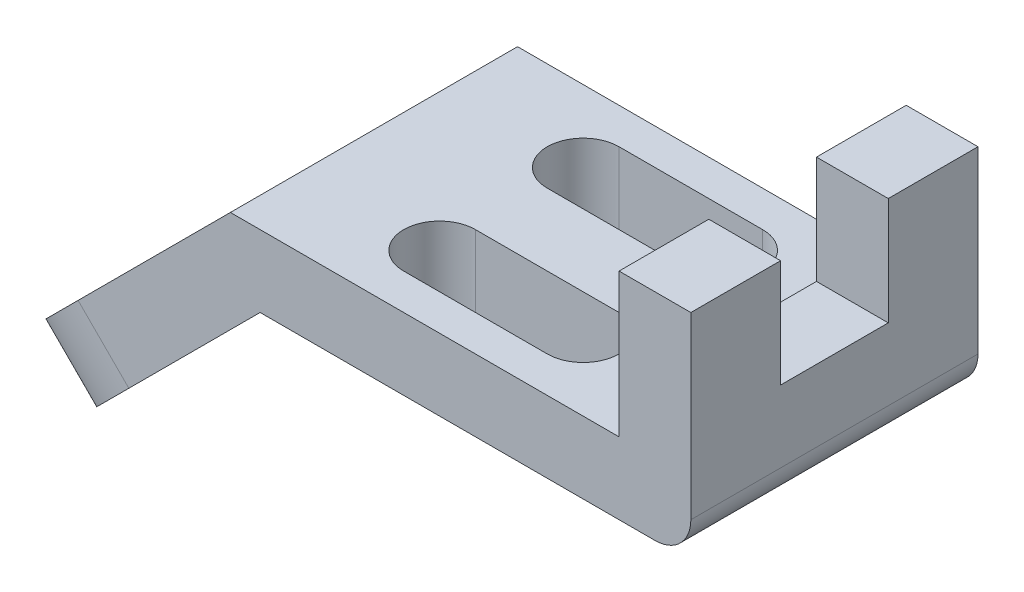
ISO-10303-21;
HEADER;
FILE_DESCRIPTION(('STEP AP214'),'2;1');
FILE_NAME('part.step','',(''),(''),'','','');
FILE_SCHEMA(('AUTOMOTIVE_DESIGN { 1 0 10303 214 1 1 1 1 }'));
ENDSEC;
DATA;
#1=APPLICATION_CONTEXT('core data for automotive mechanical design processes');
#2=APPLICATION_PROTOCOL_DEFINITION('international standard','automotive_design',2000,#1);
#3=PRODUCT_CONTEXT('',#1,'mechanical');
#4=PRODUCT('Part','Part','',(#3));
#5=PRODUCT_RELATED_PRODUCT_CATEGORY('part','',(#4));
#6=PRODUCT_DEFINITION_FORMATION('','',#4);
#7=PRODUCT_DEFINITION_CONTEXT('part definition',#1,'design');
#8=PRODUCT_DEFINITION('design','',#6,#7);
#9=PRODUCT_DEFINITION_SHAPE('','',#8);
#10=(LENGTH_UNIT() NAMED_UNIT(*) SI_UNIT(.MILLI.,.METRE.));
#11=(NAMED_UNIT(*) PLANE_ANGLE_UNIT() SI_UNIT($,.RADIAN.));
#12=(NAMED_UNIT(*) SI_UNIT($,.STERADIAN.) SOLID_ANGLE_UNIT());
#13=UNCERTAINTY_MEASURE_WITH_UNIT(LENGTH_MEASURE(1.E-05),#10,'distance_accuracy_value','');
#14=(GEOMETRIC_REPRESENTATION_CONTEXT(3) GLOBAL_UNCERTAINTY_ASSIGNED_CONTEXT((#13)) GLOBAL_UNIT_ASSIGNED_CONTEXT((#10,
#11,#12)) REPRESENTATION_CONTEXT('',''));
#15=CARTESIAN_POINT('',(0.,0.,0.));
#16=DIRECTION('',(0.,0.,1.));
#17=DIRECTION('',(1.,0.,0.));
#18=AXIS2_PLACEMENT_3D('',#15,#16,#17);
#19=CARTESIAN_POINT('',(-78.2842712474619,-18.2842712474619,0.));
#20=DIRECTION('',(-0.707106781186549,0.707106781186546,0.));
#21=DIRECTION('',(-0.707106781186546,-0.707106781186549,0.));
#22=AXIS2_PLACEMENT_3D('',#19,#20,#21);
#23=CYLINDRICAL_SURFACE('',#22,20.);
#24=DIRECTION('',(-0.707106781186549,0.707106781186546,0.));
#25=VECTOR('',#24,1.);
#26=CARTESIAN_POINT('',(-86.9558386639541,-26.9558386639541,15.7989821533687));
#27=LINE('',#26,#25);
#28=CARTESIAN_POINT('',(-86.9558386639541,-26.9558386639541,15.7989821533687));
#29=VERTEX_POINT('',#28);
#30=CARTESIAN_POINT('',(-94.0269064758195,-19.8847708520887,15.7989821533687));
#31=VERTEX_POINT('',#30);
#32=EDGE_CURVE('E50',#29,#31,#27,.T.);
#33=ORIENTED_EDGE('',*,*,#32,.F.);
#34=CARTESIAN_POINT('',(-78.2842712474619,-18.2842712474619,0.));
#35=DIRECTION('',(-0.707106781186549,0.707106781186546,0.));
#36=DIRECTION('',(-0.707106781186546,-0.707106781186549,0.));
#37=AXIS2_PLACEMENT_3D('',#34,#35,#36);
#38=CIRCLE('',#37,20.);
#39=CARTESIAN_POINT('',(-78.2842712474619,-18.2842712474619,20.));
#40=VERTEX_POINT('',#39);
#41=EDGE_CURVE('E325',#29,#40,#38,.T.);
#42=ORIENTED_EDGE('',*,*,#41,.T.);
#43=DIRECTION('',(0.707106781186547,-0.707106781186548,0.));
#44=VECTOR('',#43,1.);
#45=CARTESIAN_POINT('',(-85.3553390593273,-11.2132034355965,20.));
#46=LINE('',#45,#44);
#47=CARTESIAN_POINT('',(-85.3553390593273,-11.2132034355965,20.));
#48=VERTEX_POINT('',#47);
#49=EDGE_CURVE('E333',#48,#40,#46,.T.);
#50=ORIENTED_EDGE('',*,*,#49,.F.);
#51=CARTESIAN_POINT('',(-85.3553390593274,-11.2132034355965,0.));
#52=DIRECTION('',(-0.707106781186549,0.707106781186546,0.));
#53=DIRECTION('',(-0.707106781186546,-0.707106781186549,0.));
#54=AXIS2_PLACEMENT_3D('',#51,#52,#53);
#55=CIRCLE('',#54,20.);
#56=EDGE_CURVE('E320',#31,#48,#55,.T.);
#57=ORIENTED_EDGE('',*,*,#56,.F.);
#58=EDGE_LOOP('',(#33,#42,#50,#57));
#59=FACE_BOUND('',#58,.T.);
#60=ADVANCED_FACE('F39',(#59),#23,.T.);
#61=CARTESIAN_POINT('',(0.,30.,20.));
#62=DIRECTION('',(0.,-1.,0.));
#63=DIRECTION('',(0.,0.,-1.));
#64=AXIS2_PLACEMENT_3D('',#61,#62,#63);
#65=PLANE('',#64);
#66=DIRECTION('',(0.,0.,-1.));
#67=VECTOR('',#66,1.);
#68=CARTESIAN_POINT('',(-10.,30.,20.));
#69=LINE('',#68,#67);
#70=CARTESIAN_POINT('',(-10.,30.,-7.5));
#71=VERTEX_POINT('',#70);
#72=CARTESIAN_POINT('',(-10.,30.,-20.));
#73=VERTEX_POINT('',#72);
#74=EDGE_CURVE('E383',#71,#73,#69,.T.);
#75=ORIENTED_EDGE('',*,*,#74,.F.);
#76=DIRECTION('',(-1.,0.,0.));
#77=VECTOR('',#76,1.);
#78=CARTESIAN_POINT('',(0.001000000000001,30.,-7.5));
#79=LINE('',#78,#77);
#80=CARTESIAN_POINT('',(0.,30.,-7.5));
#81=VERTEX_POINT('',#80);
#82=EDGE_CURVE('E308',#81,#71,#79,.T.);
#83=ORIENTED_EDGE('',*,*,#82,.F.);
#84=DIRECTION('',(0.,0.,-1.));
#85=VECTOR('',#84,1.);
#86=CARTESIAN_POINT('',(0.,30.,20.));
#87=LINE('',#86,#85);
#88=CARTESIAN_POINT('',(0.,30.,-20.));
#89=VERTEX_POINT('',#88);
#90=EDGE_CURVE('E347',#81,#89,#87,.T.);
#91=ORIENTED_EDGE('',*,*,#90,.T.);
#92=DIRECTION('',(-1.,0.,0.));
#93=VECTOR('',#92,1.);
#94=CARTESIAN_POINT('',(0.,30.,-20.));
#95=LINE('',#94,#93);
#96=EDGE_CURVE('E321',#89,#73,#95,.T.);
#97=ORIENTED_EDGE('',*,*,#96,.T.);
#98=EDGE_LOOP('',(#75,#83,#91,#97));
#99=FACE_BOUND('',#98,.T.);
#100=ADVANCED_FACE('F460',(#99),#65,.F.);
#101=CARTESIAN_POINT('',(0.,30.,20.));
#102=VERTEX_POINT('',#101);
#103=CARTESIAN_POINT('',(0.,30.,7.5));
#104=VERTEX_POINT('',#103);
#105=EDGE_CURVE('E368',#102,#104,#87,.T.);
#106=ORIENTED_EDGE('',*,*,#105,.T.);
#107=DIRECTION('',(-1.,0.,0.));
#108=VECTOR('',#107,1.);
#109=CARTESIAN_POINT('',(0.001000000000001,30.,7.5));
#110=LINE('',#109,#108);
#111=CARTESIAN_POINT('',(-10.,30.,7.5));
#112=VERTEX_POINT('',#111);
#113=EDGE_CURVE('E310',#104,#112,#110,.T.);
#114=ORIENTED_EDGE('',*,*,#113,.T.);
#115=CARTESIAN_POINT('',(-10.,30.,20.));
#116=VERTEX_POINT('',#115);
#117=EDGE_CURVE('E384',#116,#112,#69,.T.);
#118=ORIENTED_EDGE('',*,*,#117,.F.);
#119=DIRECTION('',(-1.,0.,0.));
#120=VECTOR('',#119,1.);
#121=CARTESIAN_POINT('',(0.,30.,20.));
#122=LINE('',#121,#120);
#123=EDGE_CURVE('E322',#102,#116,#122,.T.);
#124=ORIENTED_EDGE('',*,*,#123,.F.);
#125=EDGE_LOOP('',(#106,#114,#118,#124));
#126=FACE_BOUND('',#125,.T.);
#127=ADVANCED_FACE('F41',(#126),#65,.F.);
#128=CARTESIAN_POINT('',(-10.,30.,20.));
#129=DIRECTION('',(1.,0.,0.));
#130=DIRECTION('',(0.,1.,0.));
#131=AXIS2_PLACEMENT_3D('',#128,#129,#130);
#132=PLANE('',#131);
#133=DIRECTION('',(0.,0.,1.));
#134=VECTOR('',#133,1.);
#135=CARTESIAN_POINT('',(-10.,15.,-7.5));
#136=LINE('',#135,#134);
#137=CARTESIAN_POINT('',(-10.,15.,-7.5));
#138=VERTEX_POINT('',#137);
#139=CARTESIAN_POINT('',(-10.,15.,7.5));
#140=VERTEX_POINT('',#139);
#141=EDGE_CURVE('E296',#138,#140,#136,.T.);
#142=ORIENTED_EDGE('',*,*,#141,.F.);
#143=DIRECTION('',(0.,-1.,0.));
#144=VECTOR('',#143,1.);
#145=CARTESIAN_POINT('',(-10.,30.,-7.5));
#146=LINE('',#145,#144);
#147=EDGE_CURVE('E299',#71,#138,#146,.T.);
#148=ORIENTED_EDGE('',*,*,#147,.F.);
#149=ORIENTED_EDGE('',*,*,#74,.T.);
#150=DIRECTION('',(0.,-1.,0.));
#151=VECTOR('',#150,1.);
#152=CARTESIAN_POINT('',(-10.,30.,-20.));
#153=LINE('',#152,#151);
#154=CARTESIAN_POINT('',(-10.,10.,-20.));
#155=VERTEX_POINT('',#154);
#156=EDGE_CURVE('E349',#73,#155,#153,.T.);
#157=ORIENTED_EDGE('',*,*,#156,.T.);
#158=DIRECTION('',(0.,0.,-1.));
#159=VECTOR('',#158,1.);
#160=CARTESIAN_POINT('',(-10.,10.,20.));
#161=LINE('',#160,#159);
#162=CARTESIAN_POINT('',(-10.,10.,20.));
#163=VERTEX_POINT('',#162);
#164=EDGE_CURVE('E381',#163,#155,#161,.T.);
#165=ORIENTED_EDGE('',*,*,#164,.F.);
#166=DIRECTION('',(0.,-1.,0.));
#167=VECTOR('',#166,1.);
#168=CARTESIAN_POINT('',(-10.,30.,20.));
#169=LINE('',#168,#167);
#170=EDGE_CURVE('E330',#116,#163,#169,.T.);
#171=ORIENTED_EDGE('',*,*,#170,.F.);
#172=ORIENTED_EDGE('',*,*,#117,.T.);
#173=DIRECTION('',(0.,1.,0.));
#174=VECTOR('',#173,1.);
#175=CARTESIAN_POINT('',(-10.,30.,7.5));
#176=LINE('',#175,#174);
#177=EDGE_CURVE('E303',#140,#112,#176,.T.);
#178=ORIENTED_EDGE('',*,*,#177,.F.);
#179=EDGE_LOOP('',(#142,#148,#149,#157,#165,#171,#172,#178));
#180=FACE_BOUND('',#179,.T.);
#181=ADVANCED_FACE('F429',(#180),#132,.F.);
#182=CARTESIAN_POINT('',(-10.,10.,20.));
#183=DIRECTION('',(0.,-1.,0.));
#184=DIRECTION('',(1.,0.,0.));
#185=AXIS2_PLACEMENT_3D('',#182,#183,#184);
#186=PLANE('',#185);
#187=DIRECTION('',(1.,0.,0.));
#188=VECTOR('',#187,1.);
#189=CARTESIAN_POINT('',(-45.,10.,-4.99999999999999));
#190=LINE('',#189,#188);
#191=CARTESIAN_POINT('',(-45.,9.99999999999999,-4.99999999999999));
#192=VERTEX_POINT('',#191);
#193=CARTESIAN_POINT('',(-25.,10.,-4.99999999999999));
#194=VERTEX_POINT('',#193);
#195=EDGE_CURVE('E245',#192,#194,#190,.T.);
#196=ORIENTED_EDGE('',*,*,#195,.F.);
#197=CARTESIAN_POINT('',(-45.,10.,-9.99999999999999));
#198=DIRECTION('',(0.,1.,0.));
#199=DIRECTION('',(-1.,0.,0.));
#200=AXIS2_PLACEMENT_3D('',#197,#198,#199);
#201=CIRCLE('',#200,5.);
#202=CARTESIAN_POINT('',(-45.,10.,-15.));
#203=VERTEX_POINT('',#202);
#204=EDGE_CURVE('E64',#203,#192,#201,.T.);
#205=ORIENTED_EDGE('',*,*,#204,.F.);
#206=DIRECTION('',(-1.,0.,0.));
#207=VECTOR('',#206,1.);
#208=CARTESIAN_POINT('',(-45.,10.,-15.));
#209=LINE('',#208,#207);
#210=CARTESIAN_POINT('',(-25.,10.,-15.));
#211=VERTEX_POINT('',#210);
#212=EDGE_CURVE('E246',#211,#203,#209,.T.);
#213=ORIENTED_EDGE('',*,*,#212,.F.);
#214=CARTESIAN_POINT('',(-25.,10.,-9.99999999999999));
#215=DIRECTION('',(0.,1.,0.));
#216=DIRECTION('',(-1.,0.,0.));
#217=AXIS2_PLACEMENT_3D('',#214,#215,#216);
#218=CIRCLE('',#217,5.);
#219=EDGE_CURVE('E250',#194,#211,#218,.T.);
#220=ORIENTED_EDGE('',*,*,#219,.F.);
#221=EDGE_LOOP('',(#196,#205,#213,#220));
#222=FACE_BOUND('',#221,.T.);
#223=DIRECTION('',(1.,0.,0.));
#224=VECTOR('',#223,1.);
#225=CARTESIAN_POINT('',(-45.,10.,15.));
#226=LINE('',#225,#224);
#227=CARTESIAN_POINT('',(-45.,9.99999999999999,15.));
#228=VERTEX_POINT('',#227);
#229=CARTESIAN_POINT('',(-25.,10.,15.));
#230=VERTEX_POINT('',#229);
#231=EDGE_CURVE('E273',#228,#230,#226,.T.);
#232=ORIENTED_EDGE('',*,*,#231,.F.);
#233=CARTESIAN_POINT('',(-45.,10.,9.99999999999999));
#234=DIRECTION('',(0.,1.,0.));
#235=DIRECTION('',(1.,0.,0.));
#236=AXIS2_PLACEMENT_3D('',#233,#234,#235);
#237=CIRCLE('',#236,5.);
#238=CARTESIAN_POINT('',(-45.,10.,4.99999999999999));
#239=VERTEX_POINT('',#238);
#240=EDGE_CURVE('E275',#239,#228,#237,.T.);
#241=ORIENTED_EDGE('',*,*,#240,.F.);
#242=DIRECTION('',(-1.,0.,0.));
#243=VECTOR('',#242,1.);
#244=CARTESIAN_POINT('',(-45.,10.,4.99999999999999));
#245=LINE('',#244,#243);
#246=CARTESIAN_POINT('',(-25.,10.,4.99999999999999));
#247=VERTEX_POINT('',#246);
#248=EDGE_CURVE('E278',#247,#239,#245,.T.);
#249=ORIENTED_EDGE('',*,*,#248,.F.);
#250=CARTESIAN_POINT('',(-25.,10.,9.99999999999999));
#251=DIRECTION('',(0.,1.,0.));
#252=DIRECTION('',(1.,0.,0.));
#253=AXIS2_PLACEMENT_3D('',#250,#251,#252);
#254=CIRCLE('',#253,5.);
#255=EDGE_CURVE('E280',#230,#247,#254,.T.);
#256=ORIENTED_EDGE('',*,*,#255,.F.);
#257=EDGE_LOOP('',(#232,#241,#249,#256));
#258=FACE_BOUND('',#257,.T.);
#259=DIRECTION('',(-1.,0.,0.));
#260=VECTOR('',#259,1.);
#261=CARTESIAN_POINT('',(-10.,10.,-20.));
#262=LINE('',#261,#260);
#263=CARTESIAN_POINT('',(-64.142135623731,9.99999999999999,-20.));
#264=VERTEX_POINT('',#263);
#265=EDGE_CURVE('E353',#155,#264,#262,.T.);
#266=ORIENTED_EDGE('',*,*,#265,.T.);
#267=DIRECTION('',(0.,0.,-1.));
#268=VECTOR('',#267,1.);
#269=CARTESIAN_POINT('',(-64.142135623731,9.99999999999999,20.));
#270=LINE('',#269,#268);
#271=CARTESIAN_POINT('',(-64.142135623731,9.99999999999999,20.));
#272=VERTEX_POINT('',#271);
#273=EDGE_CURVE('E378',#272,#264,#270,.T.);
#274=ORIENTED_EDGE('',*,*,#273,.F.);
#275=DIRECTION('',(-1.,0.,0.));
#276=VECTOR('',#275,1.);
#277=CARTESIAN_POINT('',(-10.,10.,20.));
#278=LINE('',#277,#276);
#279=EDGE_CURVE('E329',#163,#272,#278,.T.);
#280=ORIENTED_EDGE('',*,*,#279,.F.);
#281=ORIENTED_EDGE('',*,*,#164,.T.);
#282=EDGE_LOOP('',(#266,#274,#280,#281));
#283=FACE_BOUND('',#282,.T.);
#284=ADVANCED_FACE('F432',(#222,#258,#283),#186,.F.);
#285=CARTESIAN_POINT('',(-64.142135623731,9.99999999999999,20.));
#286=DIRECTION('',(0.707106781186549,-0.707106781186546,0.));
#287=DIRECTION('',(0.707106781186546,0.707106781186549,0.));
#288=AXIS2_PLACEMENT_3D('',#285,#286,#287);
#289=PLANE('',#288);
#290=CARTESIAN_POINT('',(-85.3553390593274,-11.2132034355965,0.));
#291=DIRECTION('',(-0.707106781186549,0.707106781186546,0.));
#292=DIRECTION('',(-0.707106781186546,-0.707106781186549,0.));
#293=AXIS2_PLACEMENT_3D('',#290,#291,#292);
#294=CIRCLE('',#293,12.5);
#295=CARTESIAN_POINT('',(-90.2290634162853,-16.0869277925544,10.4280209908108));
#296=VERTEX_POINT('',#295);
#297=CARTESIAN_POINT('',(-92.7290634162853,-18.5869277925544,6.89248708487803));
#298=VERTEX_POINT('',#297);
#299=EDGE_CURVE('E212',#296,#298,#294,.T.);
#300=ORIENTED_EDGE('',*,*,#299,.F.);
#301=DIRECTION('',(0.499999999999998,0.5,-0.707106781186549));
#302=VECTOR('',#301,1.);
#303=CARTESIAN_POINT('',(-90.2290634162853,-16.0869277925544,10.4280209908108));
#304=LINE('',#303,#302);
#305=EDGE_CURVE('E211',#31,#296,#304,.T.);
#306=ORIENTED_EDGE('',*,*,#305,.F.);
#307=ORIENTED_EDGE('',*,*,#56,.T.);
#308=DIRECTION('',(-0.707106781186546,-0.707106781186549,0.));
#309=VECTOR('',#308,1.);
#310=CARTESIAN_POINT('',(-64.142135623731,9.99999999999999,20.));
#311=LINE('',#310,#309);
#312=EDGE_CURVE('E335',#272,#48,#311,.T.);
#313=ORIENTED_EDGE('',*,*,#312,.F.);
#314=ORIENTED_EDGE('',*,*,#273,.T.);
#315=DIRECTION('',(-0.707106781186546,-0.707106781186549,0.));
#316=VECTOR('',#315,1.);
#317=CARTESIAN_POINT('',(-64.142135623731,9.99999999999999,-20.));
#318=LINE('',#317,#316);
#319=CARTESIAN_POINT('',(-85.3553390593273,-11.2132034355965,-20.));
#320=VERTEX_POINT('',#319);
#321=EDGE_CURVE('E352',#264,#320,#318,.T.);
#322=ORIENTED_EDGE('',*,*,#321,.T.);
#323=CARTESIAN_POINT('',(-96.5269064758195,-22.3847708520887,12.2634482474359));
#324=VERTEX_POINT('',#323);
#325=EDGE_CURVE('E221',#320,#324,#55,.T.);
#326=ORIENTED_EDGE('',*,*,#325,.T.);
#327=DIRECTION('',(-0.499999999999999,-0.5,0.707106781186549));
#328=VECTOR('',#327,1.);
#329=CARTESIAN_POINT('',(-92.7290634162853,-18.5869277925544,6.89248708487803));
#330=LINE('',#329,#328);
#331=EDGE_CURVE('E53',#298,#324,#330,.T.);
#332=ORIENTED_EDGE('',*,*,#331,.F.);
#333=EDGE_LOOP('',(#300,#306,#307,#313,#314,#322,#326,#332));
#334=FACE_BOUND('',#333,.T.);
#335=ADVANCED_FACE('F225',(#334),#289,.F.);
#336=CARTESIAN_POINT('',(-78.2842712474619,-18.2842712474619,20.));
#337=DIRECTION('',(-0.707106781186548,0.707106781186547,0.));
#338=DIRECTION('',(-0.707106781186547,-0.707106781186548,0.));
#339=AXIS2_PLACEMENT_3D('',#336,#337,#338);
#340=PLANE('',#339);
#341=ORIENTED_EDGE('',*,*,#41,.F.);
#342=DIRECTION('',(0.499999999999998,0.499999999999999,-0.707106781186549));
#343=VECTOR('',#342,1.);
#344=CARTESIAN_POINT('',(-84.1053390593273,-24.1053390593274,11.7677669529664));
#345=LINE('',#344,#343);
#346=CARTESIAN_POINT('',(-83.1579956044198,-23.1579956044199,10.4280209908108));
#347=VERTEX_POINT('',#346);
#348=EDGE_CURVE('E226',#29,#347,#345,.T.);
#349=ORIENTED_EDGE('',*,*,#348,.T.);
#350=CARTESIAN_POINT('',(-78.2842712474619,-18.2842712474619,0.));
#351=DIRECTION('',(-0.707106781186548,0.707106781186547,0.));
#352=DIRECTION('',(-0.707106781186547,-0.707106781186548,0.));
#353=AXIS2_PLACEMENT_3D('',#350,#351,#352);
#354=CIRCLE('',#353,12.5);
#355=CARTESIAN_POINT('',(-85.6579956044198,-25.6579956044199,6.89248708487803));
#356=VERTEX_POINT('',#355);
#357=EDGE_CURVE('E11',#347,#356,#354,.T.);
#358=ORIENTED_EDGE('',*,*,#357,.T.);
#359=DIRECTION('',(-0.499999999999999,-0.5,0.707106781186549));
#360=VECTOR('',#359,1.);
#361=CARTESIAN_POINT('',(-86.6053390593273,-26.6053390593274,8.23223304703367));
#362=LINE('',#361,#360);
#363=CARTESIAN_POINT('',(-89.4558386639541,-29.4558386639542,12.2634482474359));
#364=VERTEX_POINT('',#363);
#365=EDGE_CURVE('E208',#356,#364,#362,.T.);
#366=ORIENTED_EDGE('',*,*,#365,.T.);
#367=CARTESIAN_POINT('',(-78.2842712474619,-18.2842712474619,-20.));
#368=VERTEX_POINT('',#367);
#369=EDGE_CURVE('E318',#368,#364,#38,.T.);
#370=ORIENTED_EDGE('',*,*,#369,.F.);
#371=DIRECTION('',(0.707106781186547,0.707106781186548,0.));
#372=VECTOR('',#371,1.);
#373=CARTESIAN_POINT('',(-78.2842712474619,-18.2842712474619,-20.));
#374=LINE('',#373,#372);
#375=CARTESIAN_POINT('',(-60.,0.,-20.));
#376=VERTEX_POINT('',#375);
#377=EDGE_CURVE('E358',#368,#376,#374,.T.);
#378=ORIENTED_EDGE('',*,*,#377,.T.);
#379=DIRECTION('',(0.,0.,-1.));
#380=VECTOR('',#379,1.);
#381=CARTESIAN_POINT('',(-60.,0.,20.));
#382=LINE('',#381,#380);
#383=CARTESIAN_POINT('',(-60.,0.,20.));
#384=VERTEX_POINT('',#383);
#385=EDGE_CURVE('E374',#384,#376,#382,.T.);
#386=ORIENTED_EDGE('',*,*,#385,.F.);
#387=DIRECTION('',(0.707106781186547,0.707106781186548,0.));
#388=VECTOR('',#387,1.);
#389=CARTESIAN_POINT('',(-78.2842712474619,-18.2842712474619,20.));
#390=LINE('',#389,#388);
#391=EDGE_CURVE('E337',#40,#384,#390,.T.);
#392=ORIENTED_EDGE('',*,*,#391,.F.);
#393=EDGE_LOOP('',(#341,#349,#358,#366,#370,#378,#386,#392));
#394=FACE_BOUND('',#393,.T.);
#395=ADVANCED_FACE('F405',(#394),#340,.F.);
#396=CARTESIAN_POINT('',(-60.,0.,20.));
#397=DIRECTION('',(0.,1.,0.));
#398=DIRECTION('',(0.,0.,1.));
#399=AXIS2_PLACEMENT_3D('',#396,#397,#398);
#400=PLANE('',#399);
#401=DIRECTION('',(1.,0.,0.));
#402=VECTOR('',#401,1.);
#403=CARTESIAN_POINT('',(-45.,0.,-15.));
#404=LINE('',#403,#402);
#405=CARTESIAN_POINT('',(-45.,0.,-15.));
#406=VERTEX_POINT('',#405);
#407=CARTESIAN_POINT('',(-25.,0.,-15.));
#408=VERTEX_POINT('',#407);
#409=EDGE_CURVE('E237',#406,#408,#404,.T.);
#410=ORIENTED_EDGE('',*,*,#409,.F.);
#411=CARTESIAN_POINT('',(-45.,0.,-9.99999999999999));
#412=DIRECTION('',(0.,1.,0.));
#413=DIRECTION('',(0.,0.,1.));
#414=AXIS2_PLACEMENT_3D('',#411,#412,#413);
#415=CIRCLE('',#414,5.);
#416=CARTESIAN_POINT('',(-45.,0.,-4.99999999999999));
#417=VERTEX_POINT('',#416);
#418=EDGE_CURVE('E238',#417,#406,#415,.F.);
#419=ORIENTED_EDGE('',*,*,#418,.F.);
#420=DIRECTION('',(-1.,0.,0.));
#421=VECTOR('',#420,1.);
#422=CARTESIAN_POINT('',(-45.,0.,-4.99999999999999));
#423=LINE('',#422,#421);
#424=CARTESIAN_POINT('',(-25.,0.,-4.99999999999999));
#425=VERTEX_POINT('',#424);
#426=EDGE_CURVE('E258',#425,#417,#423,.T.);
#427=ORIENTED_EDGE('',*,*,#426,.F.);
#428=CARTESIAN_POINT('',(-25.,0.,-9.99999999999999));
#429=DIRECTION('',(0.,1.,0.));
#430=DIRECTION('',(0.,0.,1.));
#431=AXIS2_PLACEMENT_3D('',#428,#429,#430);
#432=CIRCLE('',#431,5.);
#433=EDGE_CURVE('E234',#408,#425,#432,.F.);
#434=ORIENTED_EDGE('',*,*,#433,.F.);
#435=EDGE_LOOP('',(#410,#419,#427,#434));
#436=FACE_BOUND('',#435,.T.);
#437=DIRECTION('',(1.,0.,0.));
#438=VECTOR('',#437,1.);
#439=CARTESIAN_POINT('',(-45.,0.,4.99999999999999));
#440=LINE('',#439,#438);
#441=CARTESIAN_POINT('',(-45.,0.,4.99999999999999));
#442=VERTEX_POINT('',#441);
#443=CARTESIAN_POINT('',(-25.,0.,4.99999999999999));
#444=VERTEX_POINT('',#443);
#445=EDGE_CURVE('E266',#442,#444,#440,.T.);
#446=ORIENTED_EDGE('',*,*,#445,.F.);
#447=CARTESIAN_POINT('',(-45.,0.,9.99999999999999));
#448=DIRECTION('',(0.,1.,0.));
#449=DIRECTION('',(0.,0.,1.));
#450=AXIS2_PLACEMENT_3D('',#447,#448,#449);
#451=CIRCLE('',#450,5.);
#452=CARTESIAN_POINT('',(-45.,0.,15.));
#453=VERTEX_POINT('',#452);
#454=EDGE_CURVE('E267',#453,#442,#451,.F.);
#455=ORIENTED_EDGE('',*,*,#454,.F.);
#456=DIRECTION('',(-1.,0.,0.));
#457=VECTOR('',#456,1.);
#458=CARTESIAN_POINT('',(-45.,0.,15.));
#459=LINE('',#458,#457);
#460=CARTESIAN_POINT('',(-25.,0.,15.));
#461=VERTEX_POINT('',#460);
#462=EDGE_CURVE('E240',#461,#453,#459,.T.);
#463=ORIENTED_EDGE('',*,*,#462,.F.);
#464=CARTESIAN_POINT('',(-25.,0.,9.99999999999999));
#465=DIRECTION('',(0.,1.,0.));
#466=DIRECTION('',(0.,0.,1.));
#467=AXIS2_PLACEMENT_3D('',#464,#465,#466);
#468=CIRCLE('',#467,5.);
#469=EDGE_CURVE('E233',#444,#461,#468,.F.);
#470=ORIENTED_EDGE('',*,*,#469,.F.);
#471=EDGE_LOOP('',(#446,#455,#463,#470));
#472=FACE_BOUND('',#471,.T.);
#473=DIRECTION('',(1.,0.,0.));
#474=VECTOR('',#473,1.);
#475=CARTESIAN_POINT('',(-60.,0.,-20.));
#476=LINE('',#475,#474);
#477=CARTESIAN_POINT('',(-5.,0.,-20.));
#478=VERTEX_POINT('',#477);
#479=EDGE_CURVE('E356',#376,#478,#476,.T.);
#480=ORIENTED_EDGE('',*,*,#479,.T.);
#481=DIRECTION('',(0.,0.,-1.));
#482=VECTOR('',#481,1.);
#483=CARTESIAN_POINT('',(-5.,0.,20.));
#484=LINE('',#483,#482);
#485=CARTESIAN_POINT('',(-5.,0.,20.));
#486=VERTEX_POINT('',#485);
#487=EDGE_CURVE('E375',#486,#478,#484,.T.);
#488=ORIENTED_EDGE('',*,*,#487,.F.);
#489=DIRECTION('',(1.,0.,0.));
#490=VECTOR('',#489,1.);
#491=CARTESIAN_POINT('',(-60.,0.,20.));
#492=LINE('',#491,#490);
#493=EDGE_CURVE('E336',#384,#486,#492,.T.);
#494=ORIENTED_EDGE('',*,*,#493,.F.);
#495=ORIENTED_EDGE('',*,*,#385,.T.);
#496=EDGE_LOOP('',(#480,#488,#494,#495));
#497=FACE_BOUND('',#496,.T.);
#498=ADVANCED_FACE('F407',(#436,#472,#497),#400,.F.);
#499=CARTESIAN_POINT('',(-5.,5.,20.));
#500=DIRECTION('',(0.,0.,-1.));
#501=DIRECTION('',(-1.,0.,0.));
#502=AXIS2_PLACEMENT_3D('',#499,#500,#501);
#503=CYLINDRICAL_SURFACE('',#502,5.);
#504=CARTESIAN_POINT('',(-5.,5.,-20.));
#505=DIRECTION('',(0.,0.,1.));
#506=DIRECTION('',(-1.,0.,0.));
#507=AXIS2_PLACEMENT_3D('',#504,#505,#506);
#508=CIRCLE('',#507,5.);
#509=CARTESIAN_POINT('',(0.,5.,-20.));
#510=VERTEX_POINT('',#509);
#511=EDGE_CURVE('E362',#478,#510,#508,.T.);
#512=ORIENTED_EDGE('',*,*,#511,.T.);
#513=DIRECTION('',(0.,0.,-1.));
#514=VECTOR('',#513,1.);
#515=CARTESIAN_POINT('',(0.,5.,20.));
#516=LINE('',#515,#514);
#517=CARTESIAN_POINT('',(0.,5.,20.));
#518=VERTEX_POINT('',#517);
#519=EDGE_CURVE('E369',#518,#510,#516,.T.);
#520=ORIENTED_EDGE('',*,*,#519,.F.);
#521=CARTESIAN_POINT('',(-5.,5.,20.));
#522=DIRECTION('',(0.,0.,1.));
#523=DIRECTION('',(-1.,0.,0.));
#524=AXIS2_PLACEMENT_3D('',#521,#522,#523);
#525=CIRCLE('',#524,5.);
#526=EDGE_CURVE('E345',#486,#518,#525,.T.);
#527=ORIENTED_EDGE('',*,*,#526,.F.);
#528=ORIENTED_EDGE('',*,*,#487,.T.);
#529=EDGE_LOOP('',(#512,#520,#527,#528));
#530=FACE_BOUND('',#529,.T.);
#531=ADVANCED_FACE('F414',(#530),#503,.T.);
#532=CARTESIAN_POINT('',(0.,5.,20.));
#533=DIRECTION('',(-1.,0.,0.));
#534=DIRECTION('',(0.,0.,1.));
#535=AXIS2_PLACEMENT_3D('',#532,#533,#534);
#536=PLANE('',#535);
#537=ORIENTED_EDGE('',*,*,#90,.F.);
#538=DIRECTION('',(0.,1.,0.));
#539=VECTOR('',#538,1.);
#540=CARTESIAN_POINT('',(0.,30.,-7.5));
#541=LINE('',#540,#539);
#542=CARTESIAN_POINT('',(0.,15.,-7.5));
#543=VERTEX_POINT('',#542);
#544=EDGE_CURVE('E293',#543,#81,#541,.T.);
#545=ORIENTED_EDGE('',*,*,#544,.F.);
#546=DIRECTION('',(0.,0.,-1.));
#547=VECTOR('',#546,1.);
#548=CARTESIAN_POINT('',(0.,15.,-7.5));
#549=LINE('',#548,#547);
#550=CARTESIAN_POINT('',(0.,15.,7.5));
#551=VERTEX_POINT('',#550);
#552=EDGE_CURVE('E306',#551,#543,#549,.T.);
#553=ORIENTED_EDGE('',*,*,#552,.F.);
#554=DIRECTION('',(0.,-1.,0.));
#555=VECTOR('',#554,1.);
#556=CARTESIAN_POINT('',(0.,30.,7.5));
#557=LINE('',#556,#555);
#558=EDGE_CURVE('E262',#104,#551,#557,.T.);
#559=ORIENTED_EDGE('',*,*,#558,.F.);
#560=ORIENTED_EDGE('',*,*,#105,.F.);
#561=DIRECTION('',(0.,1.,0.));
#562=VECTOR('',#561,1.);
#563=CARTESIAN_POINT('',(0.,5.,20.));
#564=LINE('',#563,#562);
#565=EDGE_CURVE('E344',#518,#102,#564,.T.);
#566=ORIENTED_EDGE('',*,*,#565,.F.);
#567=ORIENTED_EDGE('',*,*,#519,.T.);
#568=DIRECTION('',(0.,1.,0.));
#569=VECTOR('',#568,1.);
#570=CARTESIAN_POINT('',(0.,5.,-20.));
#571=LINE('',#570,#569);
#572=EDGE_CURVE('E327',#510,#89,#571,.T.);
#573=ORIENTED_EDGE('',*,*,#572,.T.);
#574=EDGE_LOOP('',(#537,#545,#553,#559,#560,#566,#567,#573));
#575=FACE_BOUND('',#574,.T.);
#576=ADVANCED_FACE('F420',(#575),#536,.F.);
#577=CARTESIAN_POINT('',(-5.,5.,20.));
#578=DIRECTION('',(0.,0.,-1.));
#579=DIRECTION('',(-1.,0.,0.));
#580=AXIS2_PLACEMENT_3D('',#577,#578,#579);
#581=PLANE('',#580);
#582=ORIENTED_EDGE('',*,*,#123,.T.);
#583=ORIENTED_EDGE('',*,*,#170,.T.);
#584=ORIENTED_EDGE('',*,*,#279,.T.);
#585=ORIENTED_EDGE('',*,*,#312,.T.);
#586=ORIENTED_EDGE('',*,*,#49,.T.);
#587=ORIENTED_EDGE('',*,*,#391,.T.);
#588=ORIENTED_EDGE('',*,*,#493,.T.);
#589=ORIENTED_EDGE('',*,*,#526,.T.);
#590=ORIENTED_EDGE('',*,*,#565,.T.);
#591=EDGE_LOOP('',(#582,#583,#584,#585,#586,#587,#588,#589,#590));
#592=FACE_BOUND('',#591,.T.);
#593=ADVANCED_FACE('F399',(#592),#581,.F.);
#594=CARTESIAN_POINT('',(-5.,5.,-20.));
#595=DIRECTION('',(0.,0.,-1.));
#596=DIRECTION('',(-1.,0.,0.));
#597=AXIS2_PLACEMENT_3D('',#594,#595,#596);
#598=PLANE('',#597);
#599=ORIENTED_EDGE('',*,*,#96,.F.);
#600=ORIENTED_EDGE('',*,*,#572,.F.);
#601=ORIENTED_EDGE('',*,*,#511,.F.);
#602=ORIENTED_EDGE('',*,*,#479,.F.);
#603=ORIENTED_EDGE('',*,*,#377,.F.);
#604=DIRECTION('',(0.707106781186547,-0.707106781186548,0.));
#605=VECTOR('',#604,1.);
#606=CARTESIAN_POINT('',(-85.3553390593273,-11.2132034355965,-20.));
#607=LINE('',#606,#605);
#608=EDGE_CURVE('E351',#320,#368,#607,.T.);
#609=ORIENTED_EDGE('',*,*,#608,.F.);
#610=ORIENTED_EDGE('',*,*,#321,.F.);
#611=ORIENTED_EDGE('',*,*,#265,.F.);
#612=ORIENTED_EDGE('',*,*,#156,.F.);
#613=EDGE_LOOP('',(#599,#600,#601,#602,#603,#609,#610,#611,#612));
#614=FACE_BOUND('',#613,.T.);
#615=ADVANCED_FACE('F438',(#614),#598,.T.);
#616=DIRECTION('',(-0.707106781186549,0.707106781186546,0.));
#617=VECTOR('',#616,1.);
#618=CARTESIAN_POINT('',(-89.4558386639541,-29.4558386639542,12.2634482474359));
#619=LINE('',#618,#617);
#620=EDGE_CURVE('E389',#324,#364,#619,.F.);
#621=ORIENTED_EDGE('',*,*,#620,.F.);
#622=ORIENTED_EDGE('',*,*,#325,.F.);
#623=ORIENTED_EDGE('',*,*,#608,.T.);
#624=ORIENTED_EDGE('',*,*,#369,.T.);
#625=EDGE_LOOP('',(#621,#622,#623,#624));
#626=FACE_BOUND('',#625,.T.);
#627=ADVANCED_FACE('F442',(#626),#23,.T.);
#628=CARTESIAN_POINT('',(0.001000000000001,30.,-7.5));
#629=DIRECTION('',(0.,0.,-1.));
#630=DIRECTION('',(0.,1.,0.));
#631=AXIS2_PLACEMENT_3D('',#628,#629,#630);
#632=PLANE('',#631);
#633=ORIENTED_EDGE('',*,*,#544,.T.);
#634=ORIENTED_EDGE('',*,*,#82,.T.);
#635=ORIENTED_EDGE('',*,*,#147,.T.);
#636=DIRECTION('',(-1.,0.,0.));
#637=VECTOR('',#636,1.);
#638=CARTESIAN_POINT('',(0.00100000000000273,15.,-7.5));
#639=LINE('',#638,#637);
#640=EDGE_CURVE('E301',#543,#138,#639,.T.);
#641=ORIENTED_EDGE('',*,*,#640,.F.);
#642=EDGE_LOOP('',(#633,#634,#635,#641));
#643=FACE_BOUND('',#642,.T.);
#644=ADVANCED_FACE('F444',(#643),#632,.F.);
#645=CARTESIAN_POINT('',(0.001000000000001,30.,7.5));
#646=DIRECTION('',(0.,0.,1.));
#647=DIRECTION('',(0.,-1.,0.));
#648=AXIS2_PLACEMENT_3D('',#645,#646,#647);
#649=PLANE('',#648);
#650=ORIENTED_EDGE('',*,*,#558,.T.);
#651=DIRECTION('',(-1.,0.,0.));
#652=VECTOR('',#651,1.);
#653=CARTESIAN_POINT('',(0.00100000000000273,15.,7.5));
#654=LINE('',#653,#652);
#655=EDGE_CURVE('E315',#551,#140,#654,.T.);
#656=ORIENTED_EDGE('',*,*,#655,.T.);
#657=ORIENTED_EDGE('',*,*,#177,.T.);
#658=ORIENTED_EDGE('',*,*,#113,.F.);
#659=EDGE_LOOP('',(#650,#656,#657,#658));
#660=FACE_BOUND('',#659,.T.);
#661=ADVANCED_FACE('F446',(#660),#649,.F.);
#662=CARTESIAN_POINT('',(0.00100000000000273,15.,-7.5));
#663=DIRECTION('',(0.,-1.,0.));
#664=DIRECTION('',(1.,0.,0.));
#665=AXIS2_PLACEMENT_3D('',#662,#663,#664);
#666=PLANE('',#665);
#667=ORIENTED_EDGE('',*,*,#552,.T.);
#668=ORIENTED_EDGE('',*,*,#640,.T.);
#669=ORIENTED_EDGE('',*,*,#141,.T.);
#670=ORIENTED_EDGE('',*,*,#655,.F.);
#671=EDGE_LOOP('',(#667,#668,#669,#670));
#672=FACE_BOUND('',#671,.T.);
#673=ADVANCED_FACE('F471',(#672),#666,.F.);
#674=CARTESIAN_POINT('',(-45.,-32.4274068711929,9.99999999999999));
#675=DIRECTION('',(0.,1.,0.));
#676=DIRECTION('',(-1.,0.,0.));
#677=AXIS2_PLACEMENT_3D('',#674,#675,#676);
#678=CYLINDRICAL_SURFACE('',#677,5.);
#679=ORIENTED_EDGE('',*,*,#454,.T.);
#680=DIRECTION('',(0.,1.,0.));
#681=VECTOR('',#680,1.);
#682=CARTESIAN_POINT('',(-45.,-32.4274068711929,4.99999999999999));
#683=LINE('',#682,#681);
#684=EDGE_CURVE('E285',#442,#239,#683,.T.);
#685=ORIENTED_EDGE('',*,*,#684,.T.);
#686=ORIENTED_EDGE('',*,*,#240,.T.);
#687=DIRECTION('',(0.,1.,0.));
#688=VECTOR('',#687,1.);
#689=CARTESIAN_POINT('',(-45.,-32.4274068711929,15.));
#690=LINE('',#689,#688);
#691=EDGE_CURVE('E282',#453,#228,#690,.T.);
#692=ORIENTED_EDGE('',*,*,#691,.F.);
#693=EDGE_LOOP('',(#679,#685,#686,#692));
#694=FACE_BOUND('',#693,.T.);
#695=ADVANCED_FACE('F481',(#694),#678,.F.);
#696=CARTESIAN_POINT('',(-45.,-32.4274068711929,4.99999999999999));
#697=DIRECTION('',(0.,0.,-1.));
#698=DIRECTION('',(-1.,0.,0.));
#699=AXIS2_PLACEMENT_3D('',#696,#697,#698);
#700=PLANE('',#699);
#701=ORIENTED_EDGE('',*,*,#445,.T.);
#702=DIRECTION('',(0.,1.,0.));
#703=VECTOR('',#702,1.);
#704=CARTESIAN_POINT('',(-25.,-32.4274068711929,4.99999999999999));
#705=LINE('',#704,#703);
#706=EDGE_CURVE('E287',#444,#247,#705,.T.);
#707=ORIENTED_EDGE('',*,*,#706,.T.);
#708=ORIENTED_EDGE('',*,*,#248,.T.);
#709=ORIENTED_EDGE('',*,*,#684,.F.);
#710=EDGE_LOOP('',(#701,#707,#708,#709));
#711=FACE_BOUND('',#710,.T.);
#712=ADVANCED_FACE('F486',(#711),#700,.F.);
#713=CARTESIAN_POINT('',(-25.,-32.4274068711929,9.99999999999999));
#714=DIRECTION('',(0.,1.,0.));
#715=DIRECTION('',(-1.,0.,0.));
#716=AXIS2_PLACEMENT_3D('',#713,#714,#715);
#717=CYLINDRICAL_SURFACE('',#716,5.);
#718=ORIENTED_EDGE('',*,*,#469,.T.);
#719=DIRECTION('',(0.,1.,0.));
#720=VECTOR('',#719,1.);
#721=CARTESIAN_POINT('',(-25.,-32.4274068711929,15.));
#722=LINE('',#721,#720);
#723=EDGE_CURVE('E288',#461,#230,#722,.T.);
#724=ORIENTED_EDGE('',*,*,#723,.T.);
#725=ORIENTED_EDGE('',*,*,#255,.T.);
#726=ORIENTED_EDGE('',*,*,#706,.F.);
#727=EDGE_LOOP('',(#718,#724,#725,#726));
#728=FACE_BOUND('',#727,.T.);
#729=ADVANCED_FACE('F495',(#728),#717,.F.);
#730=CARTESIAN_POINT('',(-45.,-32.4274068711929,15.));
#731=DIRECTION('',(0.,0.,1.));
#732=DIRECTION('',(1.,0.,0.));
#733=AXIS2_PLACEMENT_3D('',#730,#731,#732);
#734=PLANE('',#733);
#735=ORIENTED_EDGE('',*,*,#462,.T.);
#736=ORIENTED_EDGE('',*,*,#691,.T.);
#737=ORIENTED_EDGE('',*,*,#231,.T.);
#738=ORIENTED_EDGE('',*,*,#723,.F.);
#739=EDGE_LOOP('',(#735,#736,#737,#738));
#740=FACE_BOUND('',#739,.T.);
#741=ADVANCED_FACE('F488',(#740),#734,.F.);
#742=CARTESIAN_POINT('',(-45.,-32.4274068711929,-9.99999999999999));
#743=DIRECTION('',(0.,1.,0.));
#744=DIRECTION('',(-1.,0.,0.));
#745=AXIS2_PLACEMENT_3D('',#742,#743,#744);
#746=CYLINDRICAL_SURFACE('',#745,5.);
#747=ORIENTED_EDGE('',*,*,#418,.T.);
#748=DIRECTION('',(0.,1.,0.));
#749=VECTOR('',#748,1.);
#750=CARTESIAN_POINT('',(-45.,-32.4274068711929,-15.));
#751=LINE('',#750,#749);
#752=EDGE_CURVE('E255',#406,#203,#751,.T.);
#753=ORIENTED_EDGE('',*,*,#752,.T.);
#754=ORIENTED_EDGE('',*,*,#204,.T.);
#755=DIRECTION('',(0.,1.,0.));
#756=VECTOR('',#755,1.);
#757=CARTESIAN_POINT('',(-45.,-32.4274068711929,-4.99999999999999));
#758=LINE('',#757,#756);
#759=EDGE_CURVE('E251',#417,#192,#758,.T.);
#760=ORIENTED_EDGE('',*,*,#759,.F.);
#761=EDGE_LOOP('',(#747,#753,#754,#760));
#762=FACE_BOUND('',#761,.T.);
#763=ADVANCED_FACE('F491',(#762),#746,.F.);
#764=CARTESIAN_POINT('',(-45.,-32.4274068711929,-15.));
#765=DIRECTION('',(0.,0.,-1.));
#766=DIRECTION('',(-1.,0.,0.));
#767=AXIS2_PLACEMENT_3D('',#764,#765,#766);
#768=PLANE('',#767);
#769=ORIENTED_EDGE('',*,*,#409,.T.);
#770=DIRECTION('',(0.,1.,0.));
#771=VECTOR('',#770,1.);
#772=CARTESIAN_POINT('',(-25.,-32.4274068711929,-15.));
#773=LINE('',#772,#771);
#774=EDGE_CURVE('E260',#408,#211,#773,.T.);
#775=ORIENTED_EDGE('',*,*,#774,.T.);
#776=ORIENTED_EDGE('',*,*,#212,.T.);
#777=ORIENTED_EDGE('',*,*,#752,.F.);
#778=EDGE_LOOP('',(#769,#775,#776,#777));
#779=FACE_BOUND('',#778,.T.);
#780=ADVANCED_FACE('F504',(#779),#768,.F.);
#781=CARTESIAN_POINT('',(-25.,-32.4274068711929,-9.99999999999999));
#782=DIRECTION('',(0.,1.,0.));
#783=DIRECTION('',(-1.,0.,0.));
#784=AXIS2_PLACEMENT_3D('',#781,#782,#783);
#785=CYLINDRICAL_SURFACE('',#784,5.);
#786=ORIENTED_EDGE('',*,*,#433,.T.);
#787=DIRECTION('',(0.,1.,0.));
#788=VECTOR('',#787,1.);
#789=CARTESIAN_POINT('',(-25.,-32.4274068711929,-4.99999999999999));
#790=LINE('',#789,#788);
#791=EDGE_CURVE('E259',#425,#194,#790,.T.);
#792=ORIENTED_EDGE('',*,*,#791,.T.);
#793=ORIENTED_EDGE('',*,*,#219,.T.);
#794=ORIENTED_EDGE('',*,*,#774,.F.);
#795=EDGE_LOOP('',(#786,#792,#793,#794));
#796=FACE_BOUND('',#795,.T.);
#797=ADVANCED_FACE('F501',(#796),#785,.F.);
#798=CARTESIAN_POINT('',(-45.,-32.4274068711929,-4.99999999999999));
#799=DIRECTION('',(0.,0.,1.));
#800=DIRECTION('',(1.,0.,0.));
#801=AXIS2_PLACEMENT_3D('',#798,#799,#800);
#802=PLANE('',#801);
#803=ORIENTED_EDGE('',*,*,#426,.T.);
#804=ORIENTED_EDGE('',*,*,#759,.T.);
#805=ORIENTED_EDGE('',*,*,#195,.T.);
#806=ORIENTED_EDGE('',*,*,#791,.F.);
#807=EDGE_LOOP('',(#803,#804,#805,#806));
#808=FACE_BOUND('',#807,.T.);
#809=ADVANCED_FACE('F502',(#808),#802,.F.);
#810=CARTESIAN_POINT('',(-32.0710678118653,-64.4974746830583,0.));
#811=DIRECTION('',(-0.707106781186549,0.707106781186546,0.));
#812=DIRECTION('',(-0.707106781186546,-0.707106781186549,0.));
#813=AXIS2_PLACEMENT_3D('',#810,#811,#812);
#814=CYLINDRICAL_SURFACE('',#813,12.5);
#815=DIRECTION('',(-0.707106781186549,0.707106781186546,0.));
#816=VECTOR('',#815,1.);
#817=CARTESIAN_POINT('',(-36.9447921688233,-69.3711990400163,10.4280209908108));
#818=LINE('',#817,#816);
#819=EDGE_CURVE('E209',#347,#296,#818,.T.);
#820=ORIENTED_EDGE('',*,*,#819,.T.);
#821=ORIENTED_EDGE('',*,*,#299,.T.);
#822=DIRECTION('',(-0.707106781186549,0.707106781186546,0.));
#823=VECTOR('',#822,1.);
#824=CARTESIAN_POINT('',(-39.4447921688233,-71.8711990400163,6.89248708487803));
#825=LINE('',#824,#823);
#826=EDGE_CURVE('E204',#356,#298,#825,.T.);
#827=ORIENTED_EDGE('',*,*,#826,.F.);
#828=ORIENTED_EDGE('',*,*,#357,.F.);
#829=EDGE_LOOP('',(#820,#821,#827,#828));
#830=FACE_BOUND('',#829,.T.);
#831=ADVANCED_FACE('F214',(#830),#814,.F.);
#832=CARTESIAN_POINT('',(-36.9447921688233,-69.3711990400163,10.4280209908108));
#833=DIRECTION('',(0.5,0.500000000000002,0.707106781186546));
#834=DIRECTION('',(0.,-0.816496580927724,0.577350269189628));
#835=AXIS2_PLACEMENT_3D('',#832,#833,#834);
#836=PLANE('',#835);
#837=ORIENTED_EDGE('',*,*,#32,.T.);
#838=ORIENTED_EDGE('',*,*,#305,.T.);
#839=ORIENTED_EDGE('',*,*,#819,.F.);
#840=ORIENTED_EDGE('',*,*,#348,.F.);
#841=EDGE_LOOP('',(#837,#838,#839,#840));
#842=FACE_BOUND('',#841,.T.);
#843=ADVANCED_FACE('F393',(#842),#836,.F.);
#844=CARTESIAN_POINT('',(-39.4447921688233,-71.8711990400163,6.89248708487803));
#845=DIRECTION('',(-0.5,-0.500000000000002,-0.707106781186546));
#846=DIRECTION('',(0.,0.816496580927725,-0.577350269189628));
#847=AXIS2_PLACEMENT_3D('',#844,#845,#846);
#848=PLANE('',#847);
#849=ORIENTED_EDGE('',*,*,#826,.T.);
#850=ORIENTED_EDGE('',*,*,#331,.T.);
#851=ORIENTED_EDGE('',*,*,#620,.T.);
#852=ORIENTED_EDGE('',*,*,#365,.F.);
#853=EDGE_LOOP('',(#849,#850,#851,#852));
#854=FACE_BOUND('',#853,.T.);
#855=ADVANCED_FACE('F206',(#854),#848,.F.);
#856=CLOSED_SHELL('',(#60,#100,#127,#181,#284,#335,#395,#498,#531,#576,#593,#615,#627,#644,#661,
#673,#695,#712,#729,#741,#763,#780,#797,#809,#831,#843,#855));
#857=MANIFOLD_SOLID_BREP('B2',#856);
#858=ADVANCED_BREP_SHAPE_REPRESENTATION('',(#18,#857),#14);
#859=SHAPE_DEFINITION_REPRESENTATION(#9,#858);
ENDSEC;
END-ISO-10303-21;
